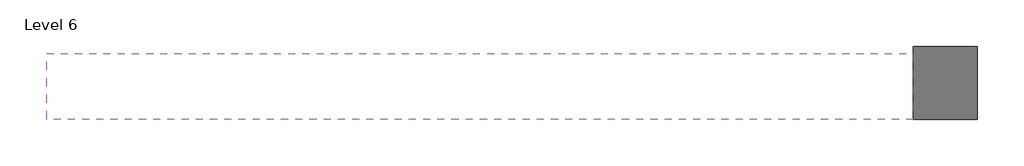
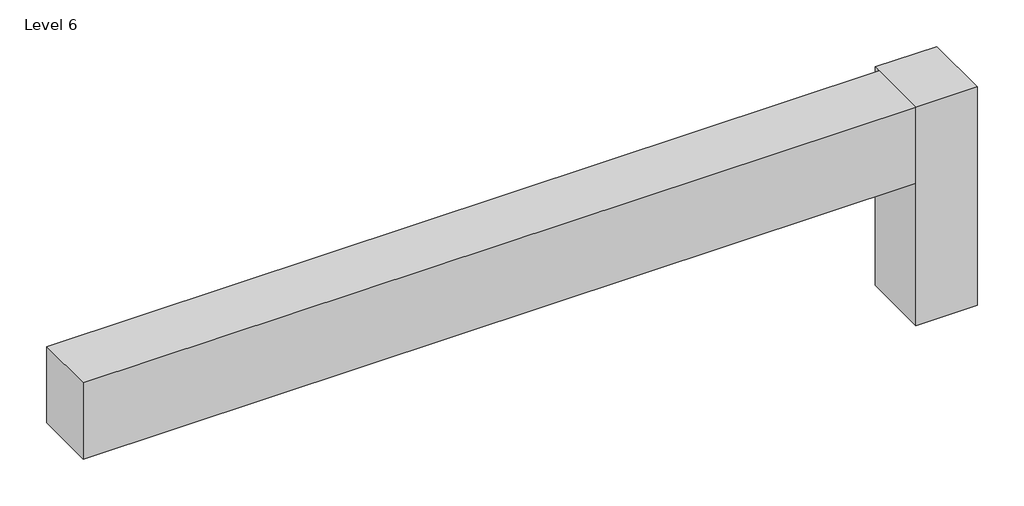
# One storey: 2 proxies.
"""IFC4 building model written with IfcOpenShell, lengths in millimetres."""

from ifc_helpers import new_model, si_unit, origin, place, context, project, spatial, transform, mapped, element, save
from components import generic_models_2_generic_models_2_1c1dda24, generic_models_3_generic_models_3_f2888e8d

model = new_model("IFC4")

# Units and contexts
model_context = context("Model", 3, world=origin())
ifc_project = project(units=[si_unit("LENGTHUNIT", "METRE", prefix="MILLI")], contexts=[model_context])

# Site, building, storey
site = spatial("IfcSite", under=ifc_project)
building = spatial("IfcBuilding", under=site)
storey = spatial("IfcBuildingStorey", under=building, Name="Level 6", Elevation=3276.6)

# Proxies
placement = place(None, origin())
generic_models_2_generic_models_2_shape = generic_models_2_generic_models_2_1c1dda24(model_context)
element("IfcBuildingElementProxy", 1, Name="Generic Models 2 : Generic Models 2", ObjectType="Generic Models 2 : Generic Models 2", at=placement, inside=storey, context=model_context, shape_type="MappedRepresentation", body=[
    mapped(generic_models_2_generic_models_2_shape, transform((0.0, 0.0, 0.0), x_axis=(1.0, 0.0, 0.0), y_axis=(0.0, 1.0, 0.0), z_axis=(0.0, 0.0, 1.0))),
])
generic_models_3_generic_models_3_shape = generic_models_3_generic_models_3_f2888e8d(model_context)
element("IfcBuildingElementProxy", 2, Name="Generic Models 3 : Generic Models 3", ObjectType="Generic Models 3 : Generic Models 3", at=placement, inside=storey, context=model_context, shape_type="MappedRepresentation", body=[
    mapped(generic_models_3_generic_models_3_shape, transform((0.0, 0.0, 0.0), x_axis=(1.0, 0.0, 0.0), y_axis=(0.0, 1.0, 0.0), z_axis=(0.0, 0.0, 1.0))),
])

save(model, "model.ifc")

# Revit data of these elements
# Element 1 (IfcBuildingElementProxy, "Generic Models 2 : Generic Models 2")
#   Phase Created = New Construction
# Element 2 (IfcBuildingElementProxy, "Generic Models 3 : Generic Models 3")
#   Phase Created = New Construction
